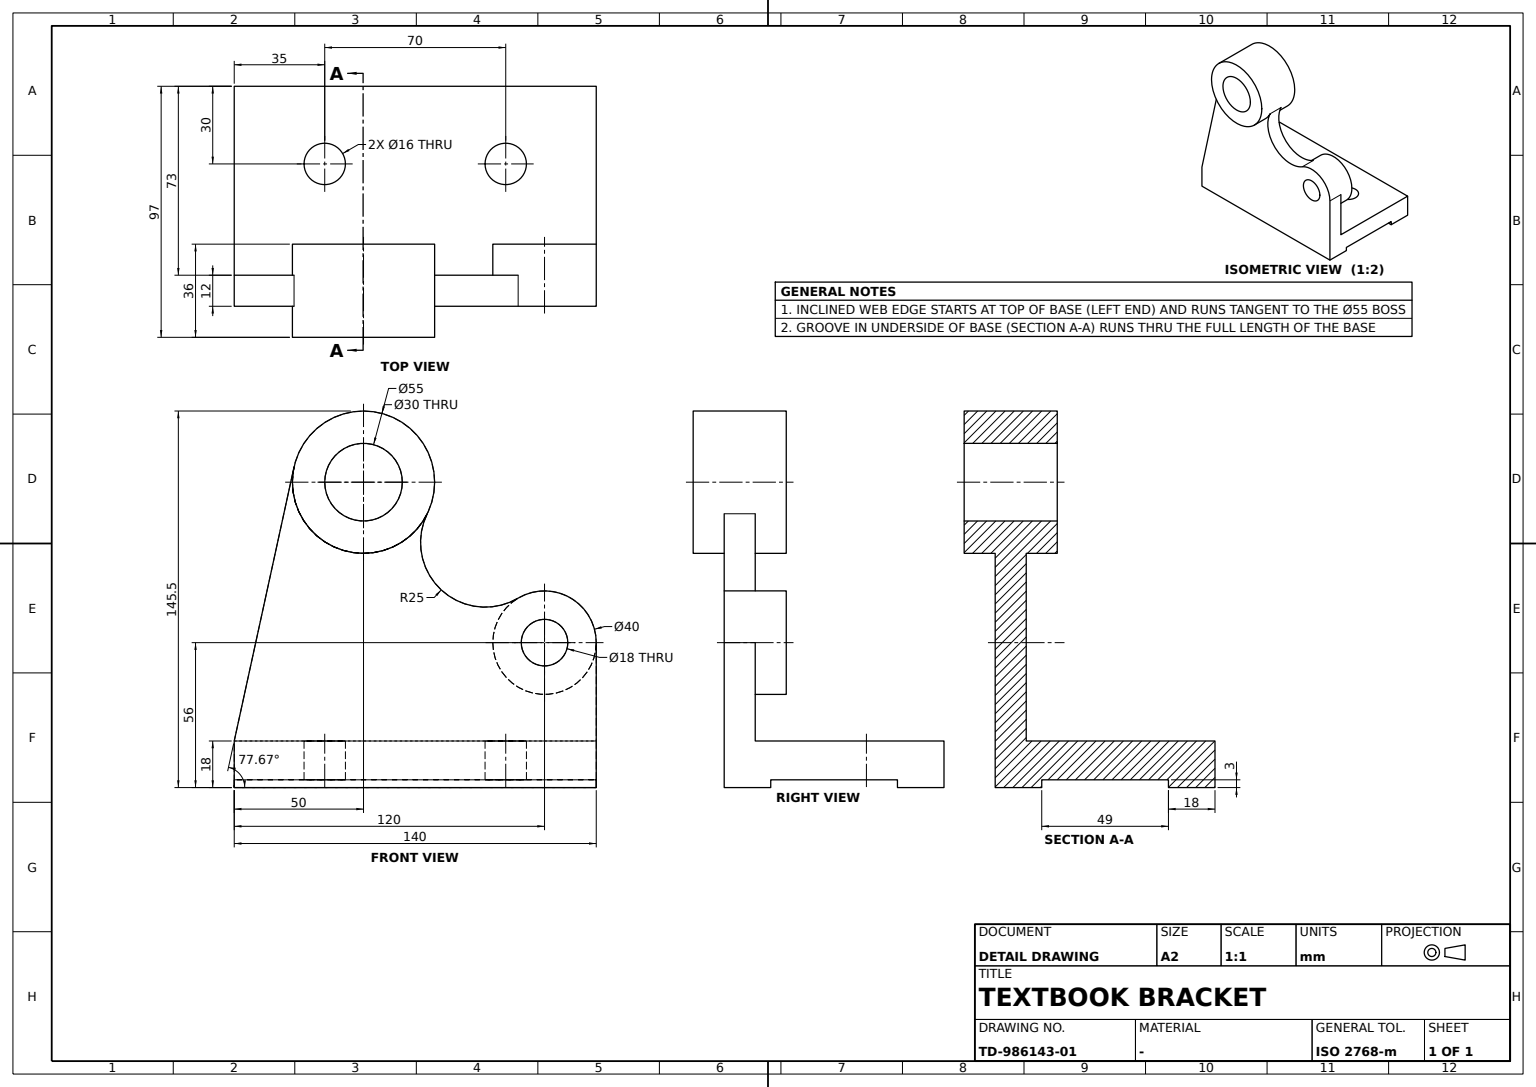
CATIA V5 part; units mm, degrees
ref_plane "Plane1" through (0, -36.5, 0) normal (0, 1, 0) x (1, 0, 0)
sketch "Sketch1" plane through (0, 0, 0) normal (1, 0, 0) x (0, 1, 0)
  line L0 (-42.5, 0) -> (42.5, 0)
  line L1 (42.5, 0) -> (42.5, -18)
  line L2 (-42.5, 0) -> (-42.5, -18)
  line L3 (-42.5, -18) -> (-24.5, -18)
  line L4 (42.5, -18) -> (24.5, -18)
  line L5 (-24.5, -18) -> (-24.5, -15)
  line L6 (-24.5, -15) -> (24.5, -15)
  line L7 (24.5, -15) -> (24.5, -18)
  dimension "length L0" = 85
  dimension "length L1" = 18
  dimension "length L3" = 18
  dimension "distance L3 L0" = 18
  dimension "length L4" = 18
  dimension "length L5" = 3
  constraint midpoint L0 origin
  constraint horizontal L0 x-axis
  constraint horizontal L3 x-axis
  constraint horizontal L4 x-axis
  constraint horizontal L6 x-axis
  constraint vertical L1 y-axis
  constraint vertical L2 y-axis
  constraint vertical L5 y-axis
  constraint vertical L7 y-axis
extrude "Pad1" add sketch "Sketch1" along normal mid plane 140
sketch "Sketch2" plane through (0, 0, 0) normal (0, 0, 1) x (1, 0, 0)
  circle A0 centre (35, 12.5) radius 8
  point P0 (35, 12.5)
  line L0 (70, 42.5) -> (70, -42.5) construction
  line L1 (-70, 42.5) -> (70, 42.5) construction
  dimension "distance P0 L0" = 35
  dimension "distance P0 L1" = 30
  dimension "radius A0" = 8
extrude "Pocket1" cut sketch "Sketch2" against normal blind 70
sketch "Sketch3" plane through (0, 0, 0) normal (0, 0, 1) x (1, 0, 0)
  circle A0 centre (-35, 12.5) radius 8
  point P0 (-35, 12.5)
  line L0 (-70, 42.5) -> (70, 42.5) construction
  line L1 (-70, 42.5) -> (-70, -42.5) construction
  dimension "radius A0" = 8
  dimension "distance P0 L0" = 30
  dimension "distance P0 L1" = 35
extrude "Pocket2" cut sketch "Sketch3" against normal blind 70
sketch "Sketch4" plane through (0, -42.5, 0) normal (0, -1, 0) x (1, 0, 0)
  circle A0 centre (50, 38) radius 20
  point P0 (50, 38)
  line L0 (-70, 0) -> (70, 0) construction
  line L1 (70, 0) -> (70, -18) construction
  dimension "radius A0" = 20
  dimension "distance P0 L0" = 38
  dimension "distance P0 L1" = 20
extrude "Pad2" add sketch "Sketch4" against normal blind 24
sketch "Sketch5" plane through (0, -18.5, 0) normal (0, 1, 0) x (-1, 0, 0)
  circle A0 centre (-50, 38) radius 9
  circle A1 centre (-50, 38) radius 20 construction
  dimension "radius A0" = 9
  constraint concentricity A0 A1
extrude "Pocket3" cut sketch "Sketch5" against normal blind 24
sketch "Sketch6" plane through (0, -36.5, 0) normal (0, -1, 0) x (1, 0, 0)
  circle A0 centre (-20, 100) radius 27.5
  point P0 (-20, 100)
  line L0 (-70, 0) -> (-70, -18) construction
  line L1 (-70, 0) -> (70, 0) construction
  dimension "radius A0" = 27.5
  dimension "distance P0 L0" = 50
  dimension "distance P0 L1" = 100
extrude "Pad3" add sketch "Sketch6" along normal mid plane 36
sketch "Sketch7" plane through (0, -42.5, 0) normal (0, -1, 0) x (1, 0, 0)
  line L0 (-70, 0) -> (70, 0)
  circle A0 centre (50, 38) radius 20 construction
  arc A1 (39.8002, 55.2036) -> (70, 38) centre (50, 38) ccw
  circle A2 centre (-20, 100) radius 27.5 construction
  arc A3 (-46.8661, 105.8705) -> (4.6454, 87.7995) centre (-20, 100) ccw
  arc A4 (4.6454, 87.7995) -> (39.8002, 55.2036) centre (27.0503, 76.7081) ccw
  point P0 (4.6454, 87.7995)
  point P1 (39.8002, 55.2036)
  line L1 (70, 0) -> (70, 38)
  point P2 (70, 38)
  line L2 (-70, 0) -> (-46.8661, 105.8705)
  point P3 (-46.8661, 105.8705)
  dimension "radius A4" = 25
  constraint coincidence A2 P0
  constraint coincidence A0 P1
  constraint coincidence A0 P2
  constraint coincidence P3 A2
  constraint tangency A4 A2
  constraint tangency A4 A0
  constraint tangency L1 A0
  constraint tangency L2 A2
extrude "Pad4" add sketch "Sketch7" against normal blind 12
sketch "Sketch8" plane through (0, -18.5, 0) normal (0, 1, 0) x (-1, 0, 0)
  circle A0 centre (20, 100) radius 15
  circle A1 centre (20, 100) radius 27.5 construction
  dimension "radius A0" = 15
  constraint concentricity A0 A1
extrude "Pocket4" cut sketch "Sketch8" against normal through all
